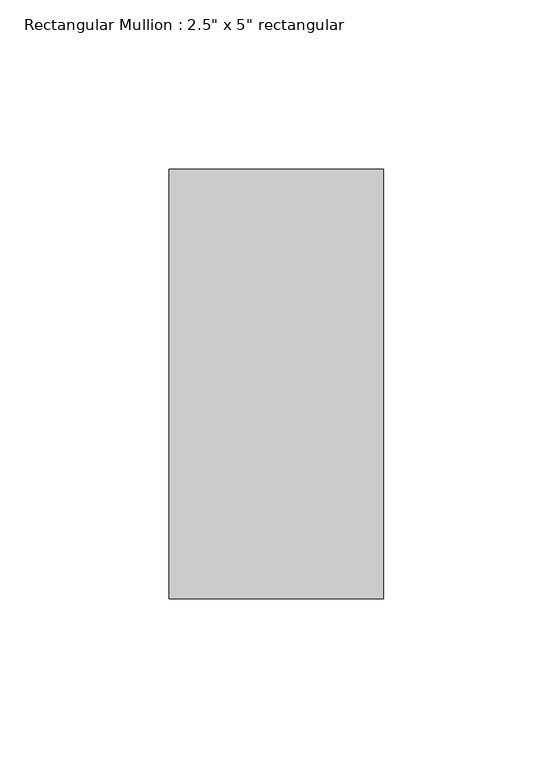
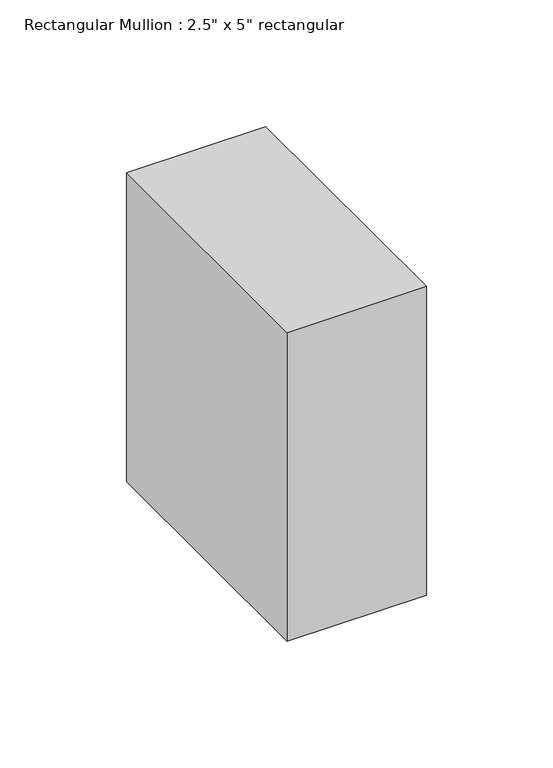
"""IFC4 building model written with IfcOpenShell, lengths in millimetres: member geometry."""

from ifc_helpers import new_model, si_unit, frame, origin, place, context, project, spatial, polyline, outline, extrude, source, transform, mapped, element, save


def member_f51719be(model_context):
    return source(origin(), model_context, "Body", "SweptSolid", [
        extrude(outline(polyline([(31.75, 63.5), (31.75, -63.5), (-31.75, -63.5), (-31.75, 63.5), (31.75, 63.5)])), frame((0.0, 0.0, -148.8191055), z_axis=(0.0, 0.0, 1.0), x_axis=(1.0, 0.0, 0.0)), (0.0, 0.0, 1.0), 148.8191055),
    ])


if __name__ == "__main__":
    model = new_model("IFC4")
    model_context = context("Model", 3, world=origin())
    ifc_project = project(units=[si_unit("LENGTHUNIT", "METRE", prefix="MILLI")], contexts=[model_context])
    site = spatial("IfcSite", under=ifc_project)
    building = spatial("IfcBuilding", under=site)
    placement = place(None, origin())
    member_shape = member_f51719be(model_context)
    element("IfcMember", 1, ObjectType="Rectangular Mullion : 2.5\" x 5\" rectangular", at=placement, inside=building, context=model_context, shape_type="MappedRepresentation", body=[
        mapped(member_shape, transform((0.0, 0.0, 0.0), x_axis=(1.0, 0.0, 0.0), y_axis=(0.0, 1.0, 0.0), z_axis=(0.0, 0.0, 1.0))),
    ])
    save(model, "model.ifc")

# Revit data of these elements
# Type "Rectangular Mullion : 2.5\" x 5\" rectangular"
#   built-in parameter 1007304 = 0.416667 (stored number, unit not read)
#   built-in parameter 1007301 = 0.104167 (stored number, unit not read)
#   built-in parameter 1007300 = 0.104167 (stored number, unit not read)
# Element 1 (IfcMember, "Rectangular Mullion : 2.5\" x 5\" rectangular")
#   Materials on its faces: "WINDOW FRAMING"
# Materials
#   "WINDOW FRAMING": class "Generic", colour RGB 120 120 120, transparency 0, Cost = 0
